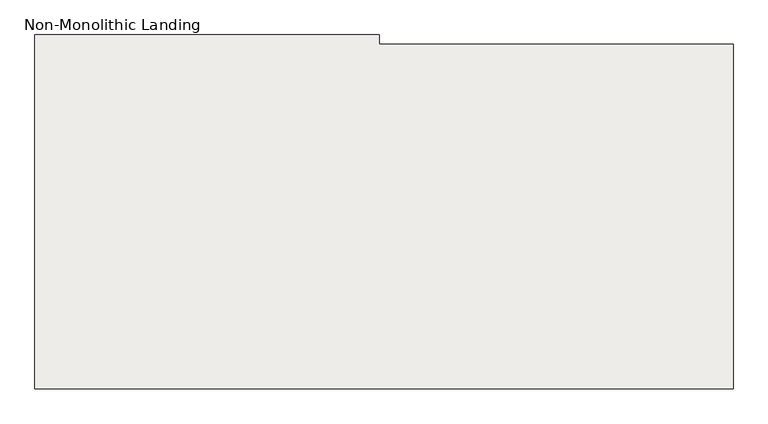
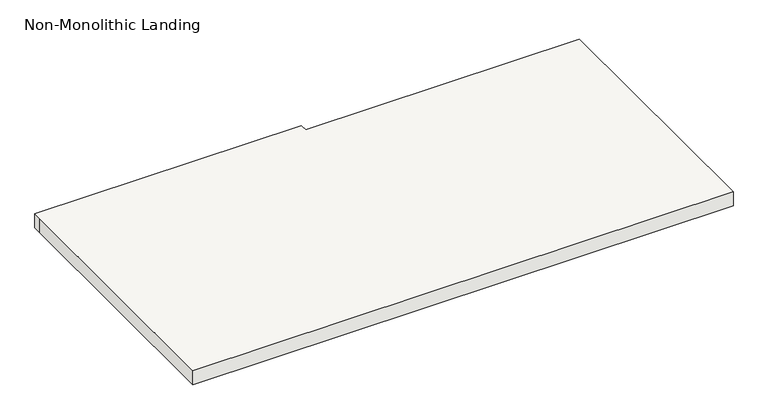
"""IFC4 building model written with IfcOpenShell, lengths in millimetres: slab geometry, Non-Monolithic Landing."""

from ifc_helpers import new_model, si_unit, origin, place, context, project, spatial, faceted_brep, source, transform, mapped, element, save


def non_monolithic_landing_f4ee6888(model_context):
    return source(origin(), model_context, "Body", "Brep", [
        faceted_brep([(-2736.9993763, -3538.5064015, 2368.55), (-2736.9993763, -3563.9064015, 2343.15), (-3651.3993763, -3563.9064015, 2343.15), (-3651.3993763, -3538.5064015, 2368.55), (-3676.7993763, -3538.5064015, 2387.6), (-3676.7993763, -3513.1064015, 2387.6), (-4591.1993763, -3513.1064015, 2387.6), (-4591.1993763, -3538.5064015, 2387.6), (-4591.1993763, -4452.9064015, 2387.6), (-2736.9993763, -4452.9064015, 2387.6), (-2736.9993763, -3538.5064015, 2387.6), (-3651.3993763, -3563.9064015, 2336.8), (-2736.9993763, -3563.9064015, 2336.8), (-2736.9993763, -4452.9064015, 2336.8), (-4591.1993763, -4452.9064015, 2336.8), (-4591.1993763, -3538.5064015, 2336.8), (-4591.1993763, -3513.1064015, 2336.8), (-3676.7993763, -3513.1064015, 2336.8), (-3676.7993763, -3538.5064015, 2336.8), (-3651.3993763, -3538.5064015, 2336.8)], [[[0, 1, 2, 3]], [[4, 5, 6, 7, 8, 9, 10]], [[11, 12, 13, 14, 15, 16, 17, 18, 19]], [[12, 11, 2, 1]], [[11, 19, 3, 2]], [[4, 10, 0, 3, 19, 18]], [[5, 4, 18, 17]], [[6, 5, 17, 16]], [[7, 6, 16, 15]], [[8, 7, 15, 14]], [[9, 8, 14, 13]], [[10, 9, 13, 12, 1, 0]]]),
    ])


if __name__ == "__main__":
    model = new_model("IFC4")
    model_context = context("Model", 3, world=origin())
    ifc_project = project(units=[si_unit("LENGTHUNIT", "METRE", prefix="MILLI")], contexts=[model_context])
    site = spatial("IfcSite", under=ifc_project)
    building = spatial("IfcBuilding", under=site)
    placement = place(None, origin())
    non_monolithic_landing_shape = non_monolithic_landing_f4ee6888(model_context)
    element("IfcSlab", 1, ObjectType="Non-Monolithic Landing", at=placement, inside=building, context=model_context, shape_type="MappedRepresentation", body=[
        mapped(non_monolithic_landing_shape, transform((0.0, 0.0, 0.0), x_axis=(1.0, 0.0, 0.0), y_axis=(0.0, 1.0, 0.0), z_axis=(0.0, 0.0, 1.0))),
    ])
    save(model, "model.ifc")
